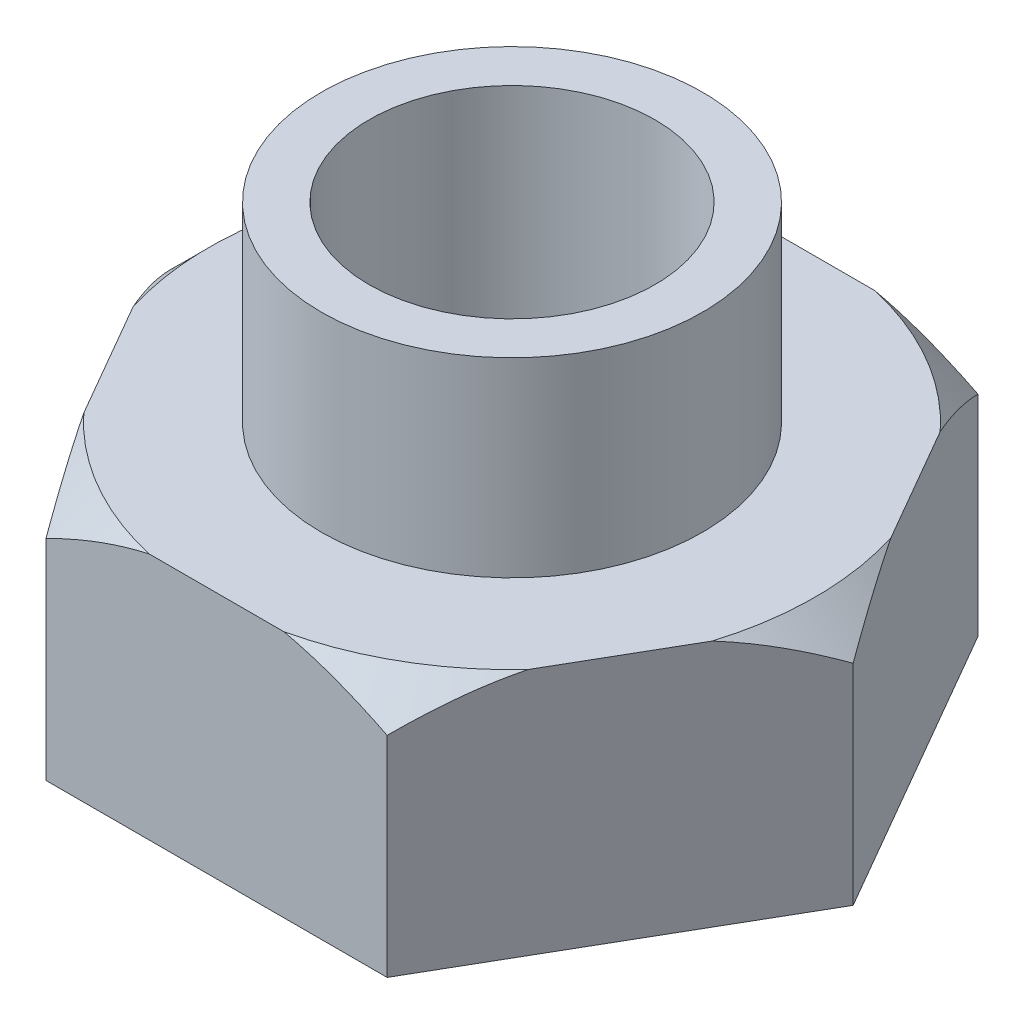
SolidWorks part; units mm, degrees
material "Titanium Ti-8Al-1Mo-1V"
ref_plane "Front Plane" through (0, 0, 0) normal (0, 0, 1) x (1, 0, 0)
ref_plane "Top Plane" through (0, 0, 0) normal (0, 1, 0) x (1, 0, 0)
ref_plane "Right Plane" through (0, 0, 0) normal (1, 0, 0) x (0, 0, -1)
sketch "Hex Profile 155AF" plane through (0, 0, 0) normal (0, 1, 0) x (1, 0, 0)
  line L1 (89.4893, 0) -> (44.7446, 77.5)
  line L2 (44.7446, 77.5) -> (-44.7446, 77.5)
  line L3 (-44.7446, 77.5) -> (-89.4893, 0)
  line L4 (-89.4893, 0) -> (-44.7446, -77.5)
  line L5 (-44.7446, -77.5) -> (44.7446, -77.5)
  line L6 (44.7446, -77.5) -> (89.4893, 0)
  circle A0 centre (0, 0) radius 77.5 construction
  dimension "D1" = 155
extrude "Hex Body 155AF x65" add sketch "Hex Profile 155AF" along normal blind 65
sketch "Hex Chamfer Profile 10x10" plane through (0, 0, 0) normal (0, 0, 1) x (1, 0, 0)
  line L0 (79.4893, 65) -> (89.4893, 65)
  line L1 (89.4893, 65) -> (89.4893, 55)
  line L2 (89.4893, 55) -> (79.4893, 65)
  line L3 (0, 0) -> (0, 65) construction
  line L4 (-44.7446, 65) -> (44.7446, 65) construction
  dimension "D1" = 10
  dimension "D2" = 10
revolve "Hex Corner Chamfer 10x10" cut sketch "Hex Chamfer Profile 10x10" angle 360 about L3
sketch "Collar Profile Ø100" plane through (0, 65, 0) normal (0, 1, 0) x (1, 0, 0)
  circle A0 centre (0, 0) radius 50
  dimension "D1" = 100
extrude "Collar Ø100 x50" add sketch "Collar Profile Ø100" along normal blind 50
sketch "Bore Profile Ø75" plane through (0, 115, 0) normal (0, 1, 0) x (1, 0, 0)
  circle A0 centre (0, 0) radius 37.5
  dimension "D1" = 75
extrude "Through Bore Ø75" cut sketch "Bore Profile Ø75" against normal up to next
